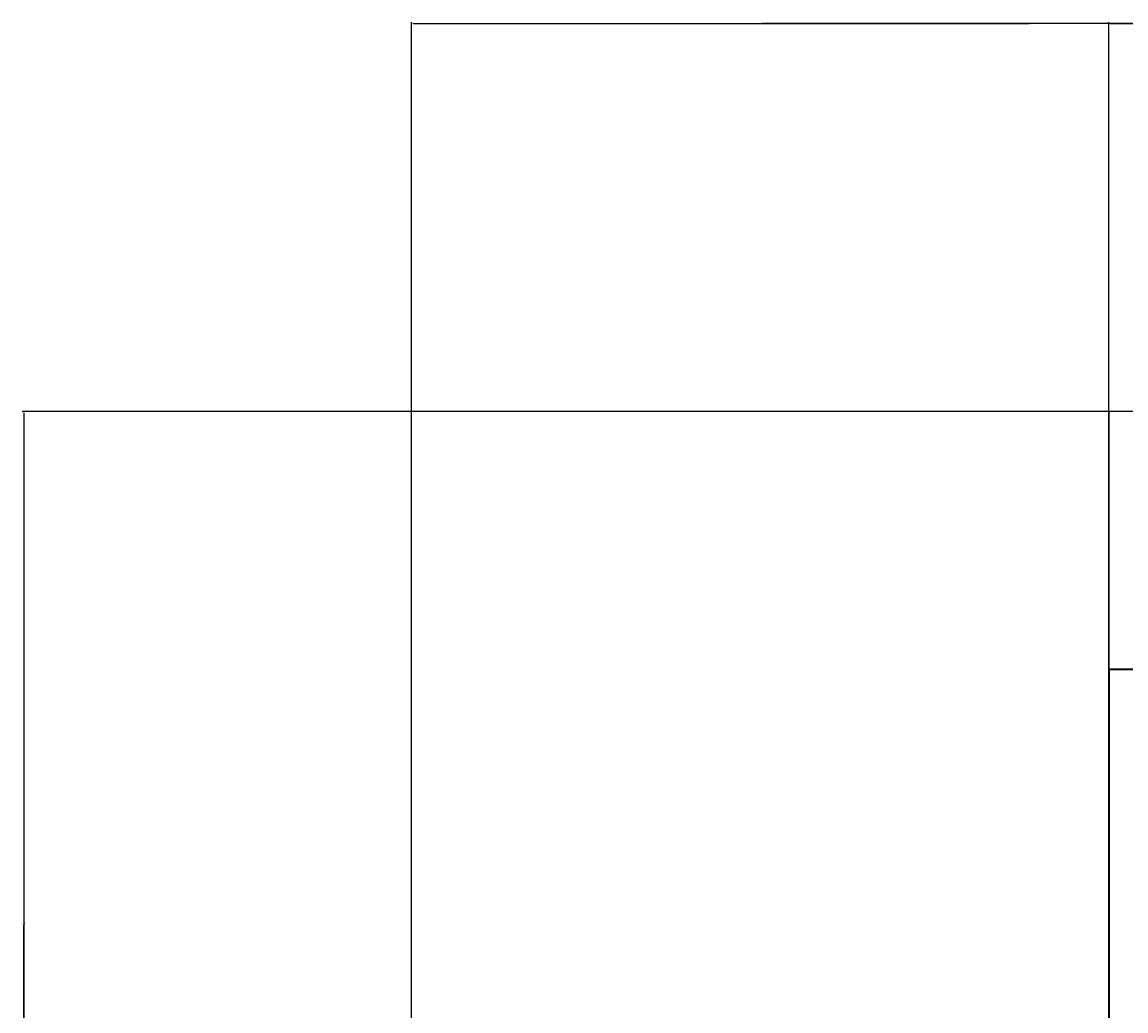
# Model space of a CAD drawing. Units: feet. Extents: x 105 to 1094, y -88 to 588.
# Tile 24 of 59: x 105 to 234, y 473 to 588. Entities that reach past the tile are written whole.
import ezdxf

# ---------------------------------------------------------------- set-up
doc = ezdxf.new("R2010")
doc.units = ezdxf.units.FT
doc.header["$MEASUREMENT"] = 0
for name, color, linetype, lineweight in [('A-ANNO-DIMS', 2, 'Continuous', 18), ('A-FLOR-PROJ', 8, 'Continuous', 25), ('A-WALL', 7, 'Continuous', 35)]:
    doc.layers.add(name, color=color, linetype=linetype, lineweight=lineweight)
doc.styles.get("Standard").update_dxf_attribs({"font": 'arial.ttf'})
doc.dimstyles.get("Standard").update_dxf_attribs({"dimtxt": 0.18, "dimasz": 0.18, "dimexe": 0.18, "dimexo": 0.0625, "dimgap": 0.09, "dimtad": 0, "dimtih": 1, "dimtoh": 1, "dimdec": 4, "dimzin": 0, "dimdsep": 46, "dimtxsty": 'Standard', "dimcen": 0.09, "dimadec": 0, "dimazin": 0, "dimtfac": 1, "dimtdec": 4, "dimtofl": 0, "dimtmove": 0, "dimatfit": 3, "dimfxl": 1, "dimtolj": 1, "dimtzin": 0, "dimarcsym": 0})

# ---------------------------------------------------------------- blocks, each defined once
blk = doc.blocks.new('*D21')
at = {"layer": 'A-ANNO-DIMS', "color": 0, "lineweight": -2, "transparency": 16777216}
for p, q in [((849.63, 543.08), (105.46, 543.08)), ((105.64, 542.9), (105.64, 250.26)), ((105.64, -42.74), (105.64, 249.9)), ((849.63, -42.92), (105.46, -42.92))]:
    blk.add_line(p, q, dxfattribs=at)
at = {"layer": 'A-ANNO-DIMS', "color": 0, "transparency": 16777216}
for points in [[(105.61, 542.9), (105.67, 542.9), (105.64, 543.08)], [(105.61, -42.74), (105.67, -42.74), (105.64, -42.92)]]:
    blk.add_solid(points, dxfattribs=at)
at = {"layer": 'Defpoints', "color": 0, "transparency": 16777216}
for p in [(105.64, 543.08), (849.69, 543.08), (849.69, -42.92)]:
    blk.add_point(p, dxfattribs=at)
at = {"layer": 'A-ANNO-DIMS', "color": 0, "transparency": 16777216, "insert": (105.64, 250.08), "char_height": 0.18, "attachment_point": 5}
blk.add_mtext('\\A1;586', dxfattribs=at)
blk = doc.blocks.new('*D22')
at = {"layer": 'A-ANNO-DIMS', "color": 0, "lineweight": -2, "transparency": 16777216}
for p, q in [((150.69, 424.14), (150.69, 588.31)), ((150.87, 588.13), (190.99, 588.13)), ((231.51, 588.13), (191.39, 588.13)), ((231.69, 543.14), (231.69, 588.31))]:
    blk.add_line(p, q, dxfattribs=at)
at = {"layer": 'A-ANNO-DIMS', "color": 0, "transparency": 16777216}
for points in [[(150.87, 588.16), (150.87, 588.1), (150.69, 588.13)], [(231.51, 588.16), (231.51, 588.1), (231.69, 588.13)]]:
    blk.add_solid(points, dxfattribs=at)
at = {"layer": 'Defpoints', "color": 0, "transparency": 16777216}
for p in [(231.69, 588.13), (231.69, 543.08), (150.69, 424.08)]:
    blk.add_point(p, dxfattribs=at)
at = {"layer": 'A-ANNO-DIMS', "color": 0, "transparency": 16777216, "insert": (191.19, 588.13), "char_height": 0.18, "attachment_point": 5}
blk.add_mtext('\\A1;81', dxfattribs=at)
blk = doc.blocks.new('*D23')
at = {"layer": 'A-ANNO-DIMS', "color": 0, "lineweight": -2, "transparency": 16777216}
for p, q in [((231.69, 543.14), (231.69, 588.31)), ((231.87, 588.13), (290.41, 588.13)), ((349.51, 588.13), (290.97, 588.13)), ((349.69, 543.14), (349.69, 588.31))]:
    blk.add_line(p, q, dxfattribs=at)
at = {"layer": 'A-ANNO-DIMS', "color": 0, "transparency": 16777216}
for points in [[(231.87, 588.16), (231.87, 588.1), (231.69, 588.13)], [(349.51, 588.16), (349.51, 588.1), (349.69, 588.13)]]:
    blk.add_solid(points, dxfattribs=at)
at = {"layer": 'Defpoints', "color": 0, "transparency": 16777216}
for p in [(349.69, 588.13), (231.69, 543.08), (349.69, 543.08)]:
    blk.add_point(p, dxfattribs=at)
at = {"layer": 'A-ANNO-DIMS', "color": 0, "transparency": 16777216, "insert": (290.69, 588.13), "char_height": 0.18, "attachment_point": 5}
blk.add_mtext('\\A1;118', dxfattribs=at)
blk = doc.blocks.new('*D27')
at = {"layer": 'A-ANNO-DIMS', "color": 0, "lineweight": -2, "transparency": 16777216}
for p, q in [((231.63, 543.08), (105.46, 543.08)), ((105.64, 542.9), (105.64, 483.76)), ((105.64, 424.26), (105.64, 483.4)), ((150.63, 424.08), (105.46, 424.08))]:
    blk.add_line(p, q, dxfattribs=at)
at = {"layer": 'A-ANNO-DIMS', "color": 0, "transparency": 16777216}
for points in [[(105.61, 542.9), (105.67, 542.9), (105.64, 543.08)], [(105.61, 424.26), (105.67, 424.26), (105.64, 424.08)]]:
    blk.add_solid(points, dxfattribs=at)
at = {"layer": 'Defpoints', "color": 0, "transparency": 16777216}
for p in [(105.64, 543.08), (231.69, 543.08), (150.69, 424.08)]:
    blk.add_point(p, dxfattribs=at)
at = {"layer": 'A-ANNO-DIMS', "color": 0, "transparency": 16777216, "insert": (105.64, 483.58), "char_height": 0.18, "attachment_point": 5}
blk.add_mtext('\\A1;119', dxfattribs=at)
blk = doc.blocks.new('*D38')
at = {"layer": 'A-ANNO-DIMS', "color": 0, "lineweight": -2, "transparency": 16777216}
for p, q in [((150.69, 224.14), (150.69, 588.31)), ((150.87, 588.13), (222.41, 588.13)), ((294.51, 588.13), (222.97, 588.13)), ((294.69, 224.14), (294.69, 588.31))]:
    blk.add_line(p, q, dxfattribs=at)
at = {"layer": 'A-ANNO-DIMS', "color": 0, "transparency": 16777216}
for points in [[(150.87, 588.16), (150.87, 588.1), (150.69, 588.13)], [(294.51, 588.16), (294.51, 588.1), (294.69, 588.13)]]:
    blk.add_solid(points, dxfattribs=at)
at = {"layer": 'Defpoints', "color": 0, "transparency": 16777216}
for p in [(294.69, 588.13), (150.69, 224.08), (294.69, 224.08)]:
    blk.add_point(p, dxfattribs=at)
at = {"layer": 'A-ANNO-DIMS', "color": 0, "transparency": 16777216, "insert": (222.69, 588.13), "char_height": 0.18, "attachment_point": 5}
blk.add_mtext('\\A1;144', dxfattribs=at)
blk = doc.blocks.new('*D42')
at = {"layer": 'A-ANNO-DIMS', "color": 0, "lineweight": -2, "transparency": 16777216}
for p, q in [((231.69, 513.14), (231.69, 588.31)), ((231.87, 588.13), (245.97, 588.13)), ((260.51, 588.13), (246.41, 588.13)), ((260.69, 513.14), (260.69, 588.31))]:
    blk.add_line(p, q, dxfattribs=at)
at = {"layer": 'A-ANNO-DIMS', "color": 0, "transparency": 16777216}
for points in [[(231.87, 588.16), (231.87, 588.1), (231.69, 588.13)], [(260.51, 588.16), (260.51, 588.1), (260.69, 588.13)]]:
    blk.add_solid(points, dxfattribs=at)
at = {"layer": 'Defpoints', "color": 0, "transparency": 16777216}
for p in [(260.69, 588.13), (231.69, 513.08), (260.69, 513.08)]:
    blk.add_point(p, dxfattribs=at)
at = {"layer": 'A-ANNO-DIMS', "color": 0, "transparency": 16777216, "insert": (246.19, 588.13), "char_height": 0.18, "attachment_point": 5}
blk.add_mtext('\\A1;29', dxfattribs=at)

msp = doc.modelspace()

# ---------------------------------------------------------------- linework, layer by layer
at = {"layer": 'A-FLOR-PROJ'}
for p, q in [((349.6883, 543.0812), (231.6883, 543.0812)), ((231.6883, 543.0812), (231.6883, 513.0812))]:
    msp.add_line(p, q, dxfattribs=at)
at = {"layer": 'A-WALL'}
for p, q in [((349.6883, 513.0812), (231.6883, 513.0812)), ((231.6883, 513.0812), (231.6883, 396.0812))]:
    msp.add_line(p, q, dxfattribs=at)

# ---------------------------------------------------------------- dimensions: what is measured, and where the dimension line sits
at = {"layer": 'A-ANNO-DIMS'}
for base, p1, p2, picture, middle in [((231.6883, 588.1312), (150.6883, 424.0812), (231.6883, 543.0812), '*D22', (191.1883, 588.1312)), ((294.6883, 588.1312), (150.6883, 224.0812), (294.6883, 224.0812), '*D38', (222.6883, 588.1312)), ((349.6883, 588.1312), (231.6883, 543.0812), (349.6883, 543.0812), '*D23', (290.6883, 588.1312)), ((260.6883, 588.1312), (231.6883, 513.0812), (260.6883, 513.0812), '*D42', (246.1883, 588.1312))]:
    dim = msp.add_linear_dim(base=base, p1=p1, p2=p2, dimstyle='Standard', override={"dimdec": 0, "dimlfac": 1, "dimrnd": 0, "dimzin": 0, "dimdsep": 46, "dimlunit": 2}, dxfattribs=at)
    dim.commit()
    dim.dimension.update_dxf_attribs({"geometry": picture, "text_midpoint": middle})
for p1, p2, picture, middle in [((849.6883, -42.9188), (849.6883, 543.0812), '*D21', (105.6383, 250.0812)), ((150.6883, 424.0812), (231.6883, 543.0812), '*D27', (105.6383, 483.5812))]:
    dim = msp.add_linear_dim(base=(105.6383, 543.0812), p1=p1, p2=p2, angle=90, dimstyle='Standard', override={"dimdec": 0, "dimlfac": 1, "dimrnd": 0, "dimzin": 0, "dimdsep": 46, "dimlunit": 2}, dxfattribs=at)
    dim.commit()
    dim.dimension.update_dxf_attribs({"geometry": picture, "text_midpoint": middle})

doc.saveas('drawing.dxf')
